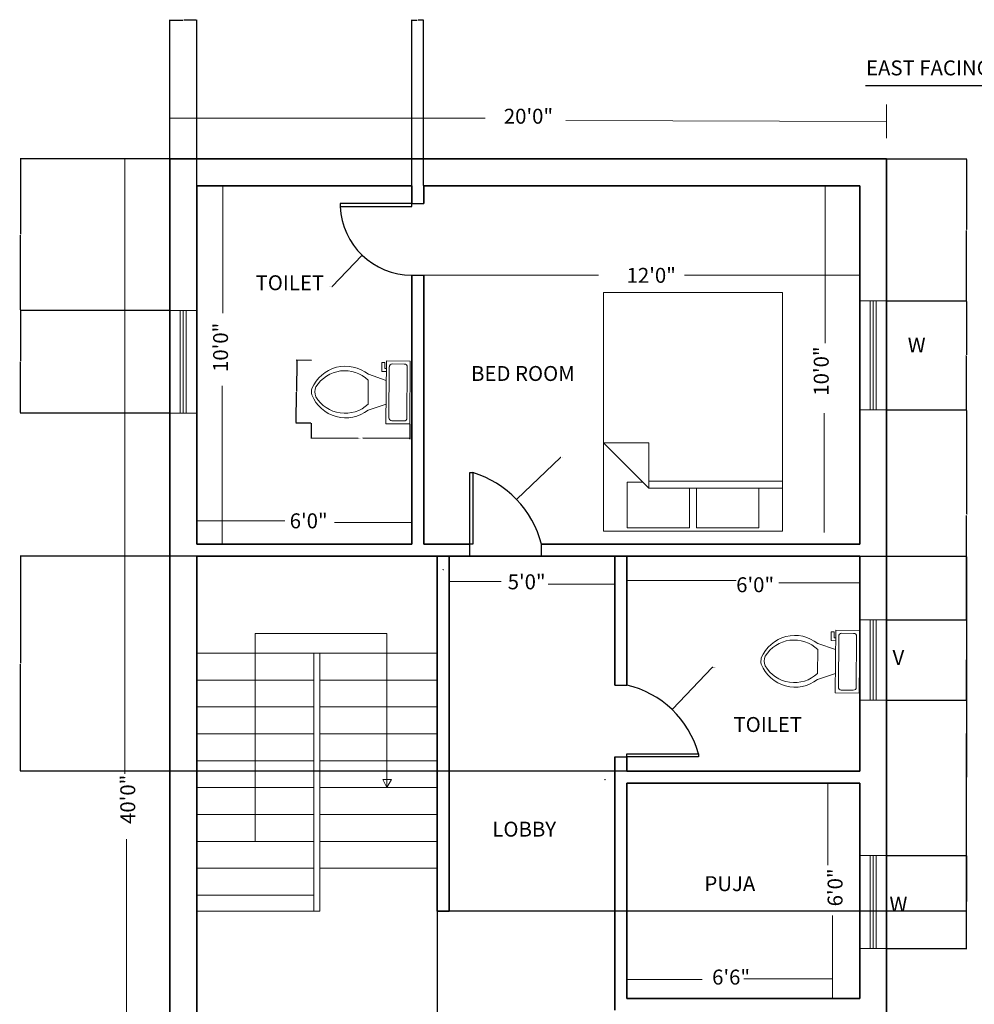
# Model space of a CAD drawing. Units: inches. Extents: x 37 to 686, y -425 to 128.
# Tile 2 of 3: x 37 to 357, y -201 to 128. Entities that reach past the tile are written whole.
import ezdxf

# ---------------------------------------------------------------- set-up
doc = ezdxf.new("R2010")
doc.units = ezdxf.units.IN
doc.header["$MEASUREMENT"] = 0
for name, color, linetype, lineweight in [('A-ANNO-DIMS', 2, 'Continuous', 13), ('A-ANNO-SYMB', 7, 'Continuous', 13), ('A-ANNO-TEXT', 7, 'Continuous', 18), ('A-ANNO-TITL', 7, 'Continuous', 25), ('A-AREA-IDEN', 7, 'Continuous', 18), ('A-DOOR', 3, 'Continuous', 25), ('A-FLOR-FIXT', 9, 'Continuous', 18), ('A-FLOR-STRS', 7, 'Continuous', 20), ('A-FURN', 8, 'Continuous', 18), ('A-GLAZ', 4, 'Continuous', 18), ('A-WALL', 7, 'Continuous', 35)]:
    doc.layers.add(name, color=color, linetype=linetype, lineweight=lineweight)
doc.styles.get("Standard").update_dxf_attribs({"font": 'arial.ttf'})
doc.dimstyles.get("Standard").update_dxf_attribs({"dimtxt": 0.18, "dimasz": 0.18, "dimexe": 0.18, "dimexo": 0.0625, "dimgap": 0.09, "dimtad": 0, "dimtih": 1, "dimtoh": 1, "dimdec": 4, "dimzin": 0, "dimdsep": 46, "dimtxsty": 'Standard', "dimcen": 0.09, "dimadec": 0, "dimazin": 0, "dimtfac": 1, "dimtdec": 4, "dimtofl": 0, "dimtmove": 0, "dimatfit": 3, "dimfxl": 1, "dimtolj": 1, "dimtzin": 0, "dimarcsym": 0})

# ---------------------------------------------------------------- blocks, each defined once
blk = doc.blocks.new('Toilet - top')
for p, q in [((9.5, -6), (9.5, -2)), ((-10, -8.5), (-8, -8.5)), ((-10, -9.5), (-10, -8.5)), ((-7, -9.5), (-10, -9.5)), ((-8, -8.5), (-8, -8)), ((-7, -8), (-7, -9.5)), ((-4, -8), (-6, -14)), ((4, -8), (6, -14)), ((4, -14), (-4, -14))]:
    blk.add_line(p, q)
blk.add_lwpolyline([(10.5, -8), (10.5, 0), (-10.5, 0), (-10.5, -8)], close=True)
for points in [[(-9.5, -2), (-9.5, -6)], [(8.5, -1), (-8.5, -1)], [(-8.5, -7), (8.5, -7)]]:
    blk.add_lwpolyline(points)
for centre, radius, start, end in [((-8.62, -1.88), 0.884, 81.8699, 188.1301), ((8.62, -1.88), 0.884, 351.8699, 98.1301), ((-8.62, -6.12), 0.884, 171.8699, 278.1301), ((8.62, -6.12), 0.884, 261.8699, 8.1301), ((3.52, -21.58), 12.17, 141.4691, 247.9714), ((4.2, -21.82), 11.33, 136.3677, 238.9468), ((-3.52, -21.58), 12.17, 292.0284, 38.5307), ((-4.2, -21.82), 11.33, 301.053, 43.6321), ((0, -27.88), 4, 245.7318, 294.2682), ((0, -29), 4, 254.8605, 285.1395)]:
    blk.add_arc(centre, radius, start, end)
blk = doc.blocks.new('Bed - Queen')
for p, q in [((0, -80.00003), (0, 0)), ((0, 0), (59.99999, 0)), ((59.99999, 0), (59.99999, -80.00003)), ((7.99999, -1.2), (28.79998, -1.2)), ((7.99999, -14.4), (7.99999, -1.2)), ((28.79998, -1.2), (28.79998, -14.4)), ((31.19999, -1.2), (51.99999, -1.2)), ((31.19999, -14.4), (31.19999, -1.2)), ((51.99999, -1.2), (51.99999, -16.4)), ((0, -14.4), (44.8, -14.4)), ((59.99999, -29.6), (44.8, -14.4)), ((44.8, -14.4), (44.8, -29.6)), ((51.99999, -16.4), (46.79936, -16.4)), ((44.8, -16.8), (0, -16.8)), ((44.8, -29.6), (59.99999, -29.6)), ((59.99999, -80.00003), (0, -80.00003))]:
    blk.add_line(p, q)
blk = doc.blocks.new('DOOR-LEAF-24IN')
for p, q in [((0, 0), (0, 24)), ((0, 24), (1, 24)), ((1, 24), (1, 0)), ((1, 0), (0, 0))]:
    blk.add_line(p, q)
blk = doc.blocks.new('*D10')
at = {"layer": 'A-ANNO-DIMS', "color": 0, "lineweight": -2, "transparency": 16777216}
for p, q in [((134.95, -6.72), (134.91, -11.8)), ((167.99, -6.97), (167.95, -12.04)), ((135.09, -11.62), (150.66, -11.73)), ((167.77, -11.86), (152.21, -11.75))]:
    blk.add_line(p, q, dxfattribs=at)
at = {"layer": 'A-ANNO-DIMS', "color": 0, "transparency": 16777216}
for points in [[(135.09, -11.59), (135.09, -11.65), (134.91, -11.62)], [(167.77, -11.83), (167.77, -11.89), (167.95, -11.86)]]:
    blk.add_solid(points, dxfattribs=at)
at = {"layer": 'Defpoints', "color": 0, "transparency": 16777216}
for p in [(134.95, -6.66), (167.99, -6.91), (167.95, -11.86)]:
    blk.add_point(p, dxfattribs=at)
at = {"layer": 'A-ANNO-DIMS', "color": 0, "transparency": 16777216, "insert": (151.43, -11.74), "char_height": 0.18, "attachment_point": 5}
blk.add_mtext('\\A1;WC 33 TYP.', dxfattribs=at)
blk = doc.blocks.new('*D11')
at = {"layer": 'A-ANNO-DIMS', "color": 0, "lineweight": -2, "transparency": 16777216}
for p, q in [((135.04, 14.34), (129.97, 14.38)), ((130.14, 14.2), (130.07, 4.06)), ((129.99, -6.44), (130.07, 3.7)), ((134.88, -6.66), (129.81, -6.62))]:
    blk.add_line(p, q, dxfattribs=at)
at = {"layer": 'A-ANNO-DIMS', "color": 0, "transparency": 16777216}
for points in [[(130.11, 14.2), (130.17, 14.2), (130.15, 14.38)], [(129.96, -6.44), (130.02, -6.44), (129.99, -6.62)]]:
    blk.add_solid(points, dxfattribs=at)
at = {"layer": 'Defpoints', "color": 0, "transparency": 16777216}
for p in [(135.1, 14.34), (129.99, -6.62), (134.95, -6.66)]:
    blk.add_point(p, dxfattribs=at)
at = {"layer": 'A-ANNO-DIMS', "color": 0, "transparency": 16777216, "insert": (130.07, 3.88), "char_height": 0.18, "attachment_point": 5}
blk.add_mtext('\\A1;21 TYP.', dxfattribs=at)
blk = doc.blocks.new('*D22')
at = {"layer": 'A-ANNO-DIMS', "color": 0, "lineweight": -2, "transparency": 16777216}
for p, q in [((240.57, -51.23), (37.48, -51.23)), ((37.66, -51.41), (37.66, -87.05)), ((37.66, -123.05), (37.66, -87.41)), ((240.57, -123.23), (37.48, -123.23))]:
    blk.add_line(p, q, dxfattribs=at)
at = {"layer": 'A-ANNO-DIMS', "color": 0, "transparency": 16777216}
for points in [[(37.63, -51.41), (37.69, -51.41), (37.66, -51.23)], [(37.63, -123.05), (37.69, -123.05), (37.66, -123.23)]]:
    blk.add_solid(points, dxfattribs=at)
at = {"layer": 'Defpoints', "color": 0, "transparency": 16777216}
for p in [(240.63, -51.23), (37.66, -123.23), (240.63, -123.23)]:
    blk.add_point(p, dxfattribs=at)
at = {"layer": 'A-ANNO-DIMS', "color": 0, "transparency": 16777216, "insert": (37.66, -87.23), "char_height": 0.18, "attachment_point": 5}
blk.add_mtext('\\A1;72', dxfattribs=at)
blk = doc.blocks.new('*D23')
at = {"layer": 'A-ANNO-DIMS', "color": 0, "lineweight": -2, "transparency": 16777216}
for p, q in [((96.63, -51.29), (96.63, -425.16)), ((177.14, -51.29), (177.14, -425.16)), ((96.81, -424.98), (136.56, -424.98)), ((176.96, -424.98), (137.21, -424.98))]:
    blk.add_line(p, q, dxfattribs=at)
at = {"layer": 'A-ANNO-DIMS', "color": 0, "transparency": 16777216}
for points in [[(96.81, -424.95), (96.81, -425.01), (96.63, -424.98)], [(176.96, -424.95), (176.96, -425.01), (177.14, -424.98)]]:
    blk.add_solid(points, dxfattribs=at)
at = {"layer": 'Defpoints', "color": 0, "transparency": 16777216}
for p in [(96.63, -51.23), (177.14, -51.23), (177.14, -424.98)]:
    blk.add_point(p, dxfattribs=at)
at = {"layer": 'A-ANNO-DIMS', "color": 0, "transparency": 16777216, "insert": (136.88, -424.98), "char_height": 0.18, "attachment_point": 5}
blk.add_mtext('\\A1;80.5', dxfattribs=at)
blk = doc.blocks.new('*D29')
at = {"layer": 'A-ANNO-DIMS', "color": 0, "lineweight": -2, "transparency": 16777216}
for p, q in [((87.57, 31.06), (37.48, 31.06)), ((37.66, 30.88), (37.66, 14.07)), ((37.66, -3.11), (37.66, 13.71)), ((87.57, -3.29), (37.48, -3.29))]:
    blk.add_line(p, q, dxfattribs=at)
at = {"layer": 'A-ANNO-DIMS', "color": 0, "transparency": 16777216}
for points in [[(37.63, 30.88), (37.69, 30.88), (37.66, 31.06)], [(37.63, -3.11), (37.69, -3.11), (37.66, -3.29)]]:
    blk.add_solid(points, dxfattribs=at)
at = {"layer": 'Defpoints', "color": 0, "transparency": 16777216}
for p in [(37.66, 31.06), (87.63, 31.06), (87.63, -3.29)]:
    blk.add_point(p, dxfattribs=at)
at = {"layer": 'A-ANNO-DIMS', "color": 0, "transparency": 16777216, "insert": (37.66, 13.89), "char_height": 0.18, "attachment_point": 5}
blk.add_mtext('\\A1;34.35', dxfattribs=at)
blk = doc.blocks.new('*D30')
at = {"layer": 'A-ANNO-DIMS', "color": 0, "lineweight": -2, "transparency": 16777216}
for p, q in [((327.69, 34.28), (354.56, 34.28)), ((354.38, 34.1), (354.38, 16.22)), ((354.38, -2.03), (354.38, 15.85)), ((327.69, -2.21), (354.56, -2.21))]:
    blk.add_line(p, q, dxfattribs=at)
at = {"layer": 'A-ANNO-DIMS', "color": 0, "transparency": 16777216}
for points in [[(354.35, 34.1), (354.41, 34.1), (354.38, 34.28)], [(354.35, -2.03), (354.41, -2.03), (354.38, -2.21)]]:
    blk.add_solid(points, dxfattribs=at)
at = {"layer": 'Defpoints', "color": 0, "transparency": 16777216}
for p in [(327.63, 34.28), (354.38, 34.28), (327.63, -2.21)]:
    blk.add_point(p, dxfattribs=at)
at = {"layer": 'A-ANNO-DIMS', "color": 0, "transparency": 16777216, "insert": (354.38, 16.03), "char_height": 0.18, "attachment_point": 5}
blk.add_mtext('\\A1;36.496', dxfattribs=at)
blk = doc.blocks.new('*D33')
at = {"layer": 'A-ANNO-DIMS', "color": 0, "lineweight": -2, "transparency": 16777216}
for p, q in [((327.69, -151.36), (354.56, -151.36)), ((354.38, -151.54), (354.38, -166.74)), ((354.38, -182.31), (354.38, -167.11)), ((327.69, -182.49), (354.56, -182.49))]:
    blk.add_line(p, q, dxfattribs=at)
at = {"layer": 'A-ANNO-DIMS', "color": 0, "transparency": 16777216}
for points in [[(354.35, -151.54), (354.41, -151.54), (354.38, -151.36)], [(354.35, -182.31), (354.41, -182.31), (354.38, -182.49)]]:
    blk.add_solid(points, dxfattribs=at)
at = {"layer": 'Defpoints', "color": 0, "transparency": 16777216}
for p in [(327.63, -151.36), (354.38, -151.36), (327.63, -182.49)]:
    blk.add_point(p, dxfattribs=at)
at = {"layer": 'A-ANNO-DIMS', "color": 0, "transparency": 16777216, "insert": (354.38, -166.92), "char_height": 0.18, "attachment_point": 5}
blk.add_mtext('\\A1;31.13', dxfattribs=at)
blk = doc.blocks.new('*D34')
at = {"layer": 'A-ANNO-DIMS', "color": 0, "lineweight": -2, "transparency": 16777216}
for p, q in [((327.69, -72.53), (354.56, -72.53)), ((354.38, -72.71), (354.38, -85.76)), ((354.38, -99.18), (354.38, -86.13)), ((327.69, -99.36), (354.56, -99.36))]:
    blk.add_line(p, q, dxfattribs=at)
at = {"layer": 'A-ANNO-DIMS', "color": 0, "transparency": 16777216}
for points in [[(354.35, -72.71), (354.41, -72.71), (354.38, -72.53)], [(354.35, -99.18), (354.41, -99.18), (354.38, -99.36)]]:
    blk.add_solid(points, dxfattribs=at)
at = {"layer": 'Defpoints', "color": 0, "transparency": 16777216}
for p in [(327.63, -72.53), (354.38, -72.53), (327.63, -99.36)]:
    blk.add_point(p, dxfattribs=at)
at = {"layer": 'A-ANNO-DIMS', "color": 0, "transparency": 16777216, "insert": (354.38, -85.94), "char_height": 0.18, "attachment_point": 5}
blk.add_mtext('\\A1;26.835', dxfattribs=at)
blk = doc.blocks.new('*D41')
at = {"layer": 'A-ANNO-DIMS', "color": 0, "lineweight": -2, "transparency": 16777216}
for p, q in [((87.57, 81.77), (37.48, 81.77)), ((37.66, 81.59), (37.66, 56.6)), ((37.66, 31.24), (37.66, 56.24)), ((87.57, 31.06), (37.48, 31.06))]:
    blk.add_line(p, q, dxfattribs=at)
at = {"layer": 'A-ANNO-DIMS', "color": 0, "transparency": 16777216}
for points in [[(37.63, 81.59), (37.69, 81.59), (37.66, 81.77)], [(37.63, 31.24), (37.69, 31.24), (37.66, 31.06)]]:
    blk.add_solid(points, dxfattribs=at)
at = {"layer": 'Defpoints', "color": 0, "transparency": 16777216}
for p in [(87.63, 81.77), (37.66, 31.06), (87.63, 31.06)]:
    blk.add_point(p, dxfattribs=at)
at = {"layer": 'A-ANNO-DIMS', "color": 0, "transparency": 16777216, "insert": (37.66, 56.42), "char_height": 0.18, "attachment_point": 5}
blk.add_mtext('\\A1;50.71', dxfattribs=at)
blk = doc.blocks.new('*D42')
at = {"layer": 'A-ANNO-DIMS', "color": 0, "lineweight": -2, "transparency": 16777216}
for p, q in [((327.69, 81.77), (354.56, 81.77)), ((354.38, 81.59), (354.38, 58.21)), ((354.38, 34.46), (354.38, 57.85)), ((327.69, 34.28), (354.56, 34.28))]:
    blk.add_line(p, q, dxfattribs=at)
at = {"layer": 'A-ANNO-DIMS', "color": 0, "transparency": 16777216}
for points in [[(354.35, 81.59), (354.41, 81.59), (354.38, 81.77)], [(354.35, 34.46), (354.41, 34.46), (354.38, 34.28)]]:
    blk.add_solid(points, dxfattribs=at)
at = {"layer": 'Defpoints', "color": 0, "transparency": 16777216}
for p in [(327.63, 81.77), (327.63, 34.28), (354.38, 34.28)]:
    blk.add_point(p, dxfattribs=at)
at = {"layer": 'A-ANNO-DIMS', "color": 0, "transparency": 16777216, "insert": (354.38, 58.03), "char_height": 0.18, "attachment_point": 5}
blk.add_mtext('\\A1;47.49', dxfattribs=at)
blk = doc.blocks.new('*D45')
at = {"layer": 'A-ANNO-DIMS', "color": 0, "lineweight": -2, "transparency": 16777216}
for p, q in [((327.69, -99.36), (354.56, -99.36)), ((354.38, -99.54), (354.38, -125.18)), ((354.38, -151.18), (354.38, -125.54)), ((327.69, -151.36), (354.56, -151.36))]:
    blk.add_line(p, q, dxfattribs=at)
at = {"layer": 'A-ANNO-DIMS', "color": 0, "transparency": 16777216}
for points in [[(354.35, -99.54), (354.41, -99.54), (354.38, -99.36)], [(354.35, -151.18), (354.41, -151.18), (354.38, -151.36)]]:
    blk.add_solid(points, dxfattribs=at)
at = {"layer": 'Defpoints', "color": 0, "transparency": 16777216}
for p in [(327.63, -99.36), (354.38, -99.36), (327.63, -151.36)]:
    blk.add_point(p, dxfattribs=at)
at = {"layer": 'A-ANNO-DIMS', "color": 0, "transparency": 16777216, "insert": (354.38, -125.36), "char_height": 0.18, "attachment_point": 5}
blk.add_mtext('\\A1;52', dxfattribs=at)
blk = doc.blocks.new('*D46')
at = {"layer": 'A-ANNO-DIMS', "color": 0, "lineweight": -2, "transparency": 16777216}
for p, q in [((327.69, -2.21), (354.56, -2.21)), ((354.38, -2.39), (354.38, -37.19)), ((354.38, -72.35), (354.38, -37.55)), ((327.69, -72.53), (354.56, -72.53))]:
    blk.add_line(p, q, dxfattribs=at)
at = {"layer": 'A-ANNO-DIMS', "color": 0, "transparency": 16777216}
for points in [[(354.35, -2.39), (354.41, -2.39), (354.38, -2.21)], [(354.35, -72.35), (354.41, -72.35), (354.38, -72.53)]]:
    blk.add_solid(points, dxfattribs=at)
at = {"layer": 'Defpoints', "color": 0, "transparency": 16777216}
for p in [(327.63, -2.21), (354.38, -2.21), (327.63, -72.53)]:
    blk.add_point(p, dxfattribs=at)
at = {"layer": 'A-ANNO-DIMS', "color": 0, "transparency": 16777216, "insert": (354.38, -37.37), "char_height": 0.18, "attachment_point": 5}
blk.add_mtext('\\A1;70.31', dxfattribs=at)
blk = doc.blocks.new('*D57')
at = {"layer": 'A-ANNO-DIMS', "color": 0, "lineweight": -2, "transparency": 16777216}
for p, q in [((177.2, -51.23), (354.56, -51.23)), ((354.38, -51.41), (354.38, -110.43)), ((354.38, -169.81), (354.38, -110.79)), ((177.2, -169.99), (354.56, -169.99))]:
    blk.add_line(p, q, dxfattribs=at)
at = {"layer": 'A-ANNO-DIMS', "color": 0, "transparency": 16777216}
for points in [[(354.35, -51.41), (354.41, -51.41), (354.38, -51.23)], [(354.35, -169.81), (354.41, -169.81), (354.38, -169.99)]]:
    blk.add_solid(points, dxfattribs=at)
at = {"layer": 'Defpoints', "color": 0, "transparency": 16777216}
for p in [(177.14, -51.23), (354.38, -51.23), (177.14, -169.99)]:
    blk.add_point(p, dxfattribs=at)
at = {"layer": 'A-ANNO-DIMS', "color": 0, "transparency": 16777216, "insert": (354.38, -110.61), "char_height": 0.18, "attachment_point": 5}
blk.add_mtext('\\A1;118.76', dxfattribs=at)
blk = doc.blocks.new('*D58')
at = {"layer": 'A-ANNO-DIMS', "color": 0, "lineweight": -2, "transparency": 16777216}
for p, q in [((87.63, 81.84), (87.63, 128.4)), ((87.81, 128.22), (91.98, 128.22)), ((96.45, 128.22), (92.28, 128.22)), ((96.63, 72.84), (96.63, 128.4))]:
    blk.add_line(p, q, dxfattribs=at)
at = {"layer": 'A-ANNO-DIMS', "color": 0, "transparency": 16777216}
for points in [[(87.81, 128.25), (87.81, 128.19), (87.63, 128.22)], [(96.45, 128.25), (96.45, 128.19), (96.63, 128.22)]]:
    blk.add_solid(points, dxfattribs=at)
at = {"layer": 'Defpoints', "color": 0, "transparency": 16777216}
for p in [(96.63, 128.22), (87.63, 81.77), (96.63, 72.77)]:
    blk.add_point(p, dxfattribs=at)
at = {"layer": 'A-ANNO-DIMS', "color": 0, "transparency": 16777216, "insert": (92.13, 128.22), "char_height": 0.18, "attachment_point": 5}
blk.add_mtext('\\A1;9', dxfattribs=at)
blk = doc.blocks.new('*D59')
at = {"layer": 'A-ANNO-DIMS', "color": 0, "lineweight": -2, "transparency": 16777216}
for p, q in [((168.63, 72.84), (168.63, 128.4)), ((168.81, 128.22), (170.48, 128.22)), ((172.45, 128.22), (170.78, 128.22)), ((172.63, 72.84), (172.63, 128.4))]:
    blk.add_line(p, q, dxfattribs=at)
at = {"layer": 'A-ANNO-DIMS', "color": 0, "transparency": 16777216}
for points in [[(168.81, 128.25), (168.81, 128.19), (168.63, 128.22)], [(172.45, 128.25), (172.45, 128.19), (172.63, 128.22)]]:
    blk.add_solid(points, dxfattribs=at)
at = {"layer": 'Defpoints', "color": 0, "transparency": 16777216}
for p in [(172.63, 128.22), (168.63, 72.77), (172.63, 72.77)]:
    blk.add_point(p, dxfattribs=at)
at = {"layer": 'A-ANNO-DIMS', "color": 0, "transparency": 16777216, "insert": (170.63, 128.22), "char_height": 0.18, "attachment_point": 5}
blk.add_mtext('\\A1;4', dxfattribs=at)
blk = doc.blocks.new('*D62')
at = {"layer": 'A-ANNO-DIMS', "color": 0, "lineweight": -2, "transparency": 16777216}
for p, q in [((218.42, -18.12), (203.84, -32.1)), ((218.6, -18.12), (218.42, -18.12)), ((179.11, -55.71), (179.29, -55.71)), ((179.2, -55.8), (179.2, -55.62))]:
    blk.add_line(p, q, dxfattribs=at)
at = {"layer": 'A-ANNO-DIMS', "color": 0, "transparency": 16777216}
blk.add_solid([(203.82, -32.07), (203.87, -32.12), (203.72, -32.22)], dxfattribs=at)
at = {"layer": 'Defpoints', "color": 0, "transparency": 16777216}
for p in [(203.72, -32.22), (179.2, -55.71)]:
    blk.add_point(p, dxfattribs=at)
at = {"layer": 'A-ANNO-DIMS', "color": 0, "transparency": 16777216, "insert": (219.08, -18.12), "char_height": 0.18, "attachment_point": 5}
blk.add_mtext('\\A1;R33.95', dxfattribs=at)
blk = doc.blocks.new('*D64')
at = {"layer": 'A-ANNO-DIMS', "color": 0, "lineweight": -2, "transparency": 16777216}
for p, q in [((269.26, -88.51), (255.93, -102.42)), ((269.44, -88.51), (269.26, -88.51)), ((233.28, -125.96), (233.46, -125.96)), ((233.37, -126.05), (233.37, -125.87))]:
    blk.add_line(p, q, dxfattribs=at)
at = {"layer": 'A-ANNO-DIMS', "color": 0, "transparency": 16777216}
blk.add_solid([(255.91, -102.4), (255.95, -102.44), (255.8, -102.55)], dxfattribs=at)
at = {"layer": 'Defpoints', "color": 0, "transparency": 16777216}
for p in [(255.8, -102.55), (233.37, -125.96)]:
    blk.add_point(p, dxfattribs=at)
at = {"layer": 'A-ANNO-DIMS', "color": 0, "transparency": 16777216, "insert": (269.92, -88.51), "char_height": 0.18, "attachment_point": 5}
blk.add_mtext('\\A1;R32.42', dxfattribs=at)
blk = doc.blocks.new('*D68')
at = {"layer": 'A-ANNO-DIMS', "color": 0, "lineweight": -2, "transparency": 16777216}
for p, q in [((168.74, 67.06), (168.92, 67.06)), ((168.83, 66.97), (168.83, 67.15)), ((142.01, 39.06), (151.94, 49.43)), ((141.83, 39.06), (142.01, 39.06))]:
    blk.add_line(p, q, dxfattribs=at)
at = {"layer": 'A-ANNO-DIMS', "color": 0, "transparency": 16777216}
blk.add_solid([(151.92, 49.45), (151.96, 49.41), (152.07, 49.56)], dxfattribs=at)
at = {"layer": 'Defpoints', "color": 0, "transparency": 16777216}
for p in [(168.83, 67.06), (152.07, 49.56)]:
    blk.add_point(p, dxfattribs=at)
at = {"layer": 'A-ANNO-DIMS', "color": 0, "transparency": 16777216, "insert": (141.28, 39.06), "char_height": 0.18, "attachment_point": 5}
blk.add_mtext('\\A1;R24.234', dxfattribs=at)

msp = doc.modelspace()

# ---------------------------------------------------------------- linework, layer by layer
at = {"layer": 'A-ANNO-DIMS'}
for p, q in [((87.6318, 89.3296), (87.6318, 101.4672)), ((327.6318, 88.7375), (327.6318, 99.987)), ((87.6318, 95.3984), (193.251, 95.3984)), ((220.2222, 94.6583), (327.6318, 94.3623)), ((80.7552, 81.7729), (64.4114, 81.7729)), ((72.5833, 81.7729), (72.5833, -124.1157)), ((105.4086, 30.1915), (105.4086, 72.7729)), ((307.0425, 72.7729), (307.0425, 30.3669)), ((172.6318, 42.8225), (231.1891, 42.8225)), ((259.9386, 42.8225), (318.6318, 42.8225)), ((307.0425, 30.3669), (307.0425, 20.1003)), ((105.1115, 5.8627), (105.1115, -47.2271)), ((306.7951, -3.3013), (306.7951, -43.2278)), ((96.6318, -39.3418), (126.118, -39.3418)), ((142.7992, -39.9243), (168.6318, -39.9243)), ((181.1379, -59.6558), (198.6356, -59.6558)), ((214.275, -60.6092), (236.6318, -60.6092)), ((240.6318, -59.3672), (277.2772, -59.3672)), ((291.6142, -60.0741), (318.6318, -60.0741)), ((307.994, -127.2271), (307.994, -154.6672)), ((73.1317, -145.9359), (73.1317, -398.2271)), ((309.5265, -171.5046), (309.5265, -199.2271)), ((240.6318, -192.9341), (265.8511, -192.9341)), ((279.8349, -192.7428), (309.5265, -192.7428))]:
    msp.add_line(p, q, dxfattribs=at)
at = {"layer": 'A-ANNO-SYMB'}
for p, q in [((116.2583, -146.6754), (116.2583, -77.1163)), ((116.2583, -77.1163), (160.3362, -77.1163)), ((160.3362, -77.1163), (160.3362, -128.6754)), ((158.9278, -125.973), (161.814, -125.973)), ((160.2537, -128.6754), (158.9278, -125.973)), ((161.814, -125.973), (160.2537, -128.6754))]:
    msp.add_line(p, q, dxfattribs=at)
at = {"layer": 'A-ANNO-TITL'}
msp.add_line((320.568, 106.3633), (393.4497, 106.3633), dxfattribs=at)
at = {"layer": 'A-DOOR'}
for p, q in [((168.6318, 66.8225), (144.6318, 66.8225)), ((144.6318, 66.8225), (144.6318, 65.8225)), ((168.6318, 65.8225), (168.6318, 67.4973)), ((168.6318, 66.8225), (172.6318, 66.8225)), ((144.6318, 65.8225), (168.6318, 65.8225)), ((168.6318, 42.8225), (172.6318, 42.8225)), ((188.0768, -51.2271), (188.0768, -47.2271)), ((212.0768, -51.2271), (212.0768, -47.2271)), ((236.6318, -94.361), (240.6318, -94.361)), ((236.6318, -118.361), (240.6318, -118.361))]:
    msp.add_line(p, q, dxfattribs=at)
for centre, radius, start, end in [((168.8344, 67.0557), 24.234, 182.916723, 269.521028), ((179.2016, -55.7117), 33.9524, 14.471364, 73.090885), ((233.3707, -125.9595), 32.4221, 15.379189, 77.058561)]:
    msp.add_arc(centre, radius, start, end, dxfattribs=at)
at = {"layer": 'A-FLOR-STRS'}
for p, q in [((177.1379, -83.6754), (96.6318, -83.6754)), ((135.8849, -169.9919), (135.8849, -83.6754)), ((137.8849, -169.9919), (137.8849, -83.6754)), ((135.8849, -92.6754), (96.6318, -92.6754)), ((177.1379, -92.6754), (137.8849, -92.6754)), ((135.8849, -101.6754), (96.6318, -101.6754)), ((177.1379, -101.6754), (137.8849, -101.6754)), ((135.8849, -110.6754), (96.6318, -110.6754)), ((177.1379, -110.6754), (137.8849, -110.6754)), ((135.8849, -119.6754), (96.6318, -119.6754)), ((177.1379, -119.6754), (137.8849, -119.6754)), ((135.8849, -128.6754), (96.6318, -128.6754)), ((177.1379, -128.6754), (137.8849, -128.6754)), ((135.8849, -137.6754), (96.6318, -137.6754)), ((177.1379, -137.6754), (137.8849, -137.6754)), ((135.8849, -146.6754), (96.6318, -146.6754)), ((177.1379, -146.6754), (137.8849, -146.6754)), ((135.8849, -155.6754), (96.6318, -155.6754)), ((177.1379, -155.6754), (137.8849, -155.6754)), ((135.8849, -164.6754), (96.6318, -164.6754)), ((137.8849, -169.9919), (96.6318, -169.9919))]:
    msp.add_line(p, q, dxfattribs=at)
at = {"layer": 'A-GLAZ'}
for p, q in [((318.6318, 34.2824), (327.6318, 34.2824)), ((322.1318, 34.2824), (322.1318, -2.2137)), ((323.1318, 34.2824), (323.1318, -2.2137)), ((324.1318, 34.2824), (324.1318, -2.2137)), ((87.6318, 31.0642), (96.6318, 31.0642)), ((91.1318, 31.0642), (91.1318, -3.2851)), ((92.1318, 31.0642), (92.1318, -3.2851)), ((93.1318, 31.0642), (93.1318, -3.2851)), ((87.6318, -3.2851), (96.6318, -3.2851)), ((318.6318, -2.2137), (327.6318, -2.2137)), ((318.6318, -72.5261), (327.6318, -72.5261)), ((322.1318, -72.5261), (322.1318, -99.3614)), ((323.1318, -72.5261), (323.1318, -99.3614)), ((324.1318, -72.5261), (324.1318, -99.3614)), ((318.6318, -99.3614), (327.6318, -99.3614)), ((318.6318, -151.3603), (327.6318, -151.3603)), ((322.1318, -151.3603), (322.1318, -182.4893)), ((323.1318, -151.3603), (323.1318, -182.4893)), ((324.1318, -151.3603), (324.1318, -182.4893)), ((318.6318, -182.4893), (327.6318, -182.4893))]:
    msp.add_line(p, q, dxfattribs=at)
at = {"layer": 'A-WALL'}
for p, q in [((96.6318, 72.7729), (168.6318, 72.7729)), ((96.6318, -47.2271), (96.6318, 72.7729)), ((168.6318, 66.8225), (168.6318, 72.7729)), ((172.6318, 66.8225), (172.6318, 72.7729)), ((172.6318, 72.7729), (318.6318, 72.7729)), ((318.6318, 72.7729), (318.6318, -47.2271)), ((168.6318, -47.2271), (168.6318, 42.8225)), ((172.6318, -47.2271), (172.6318, 42.8225)), ((96.6318, -47.2271), (168.6318, -47.2271)), ((172.6318, -47.2271), (188.0768, -47.2271)), ((212.0768, -47.2271), (318.6318, -47.2271)), ((96.6318, -389.2271), (96.6318, -51.2271)), ((96.6318, -51.2271), (177.1379, -51.2271)), ((177.1379, -51.2271), (177.1379, -153.2802)), ((181.1379, -51.2271), (181.1379, -153.2802)), ((181.1379, -51.2271), (188.0768, -51.2271)), ((212.0768, -51.2271), (236.6318, -51.2271)), ((236.6318, -51.2271), (236.6318, -94.361)), ((240.6318, -51.2271), (240.6318, -94.361)), ((240.6318, -51.2271), (318.6318, -51.2271)), ((318.6318, -51.2271), (318.6318, -123.2271)), ((236.6318, -118.361), (236.6318, -203.2271)), ((240.6318, -118.361), (240.6318, -123.2271)), ((240.6318, -123.2271), (318.6318, -123.2271)), ((240.6318, -127.2271), (318.6318, -127.2271)), ((240.6318, -127.2271), (240.6318, -199.2271)), ((318.6318, -127.2271), (318.6318, -199.2271)), ((177.1379, -153.2802), (177.1379, -169.9919)), ((181.1379, -169.9919), (181.1379, -153.2802)), ((177.1379, -169.9919), (181.1379, -169.9919)), ((240.6318, -199.2271), (318.6318, -199.2271))]:
    msp.add_line(p, q, dxfattribs=at)
msp.add_lwpolyline([(87.6318, 81.7729), (327.6318, 81.7729), (327.6318, -398.2271), (87.6318, -398.2271)], close=True, dxfattribs=at)

# ---------------------------------------------------------------- block references
at = {"layer": 'A-DOOR'}
msp.add_blockref('DOOR-LEAF-24IN', (188.077, -47.227), dxfattribs=at)
at = {"layer": 'A-DOOR', "rotation": 89.99999999999991}
msp.add_blockref('DOOR-LEAF-24IN', (264.6317, -118.3608), dxfattribs=at)
at = {"layer": 'A-FLOR-FIXT', "rotation": 269.5733184257299}
for p in [(168.0698, 3.5942), (318.5536, -86.558)]:
    msp.add_blockref('Toilet - top', p, dxfattribs=at)
at = {"layer": 'A-FURN', "rotation": 180}
msp.add_blockref('Bed - Queen', (292.8168, -42.8782), dxfattribs=at)

# ---------------------------------------------------------------- texts
at = {"layer": 'A-ANNO-DIMS', "char_height": 5, "attachment_point": 1}
for s, width, insert in [('20\'0"', 66.49393, (199.4751, 98.5799)), ('12\'0"', 35.858568, (240.5954, 45.3112)), ('6\'0"', 27.670391, (127.7758, -36.8746)), ('5\'0"', 20.747672, (200.7652, -57.2907)), ('6\'0"', 27.670391, (277.2772, -58.2717)), ('6\'6"', 30.841433, (269.2204, -189.619))]:
    msp.add_mtext_dynamic_manual_height_columns(s, width=width, gutter_width=25, heights=[0], dxfattribs=dict(at, insert=insert))
at = {"layer": 'A-ANNO-DIMS', "char_height": 5, "attachment_point": 1, "rotation": 90}
for s, width, insert in [('10\'0"', 27.842625, (102.1156, 10.4667)), ('10\'0"', 27.842625, (303.2568, 2.5243)), ('40\'0"', 31.535776, (71.0496, -140.8477)), ('6\'0"', 27.670391, (307.9005, -168.4409))]:
    msp.add_mtext_dynamic_manual_height_columns(s, width=width, gutter_width=25, heights=[0], dxfattribs=dict(at, insert=insert))
at = {"layer": 'A-ANNO-TEXT', "char_height": 5, "attachment_point": 1}
for s, width, insert in [('W', 14.305566, (334.722, 22.0003)), ('V', 13.447234, (329.6363, -82.6031)), ('W', 8.568355, (328.6141, -165.2002))]:
    msp.add_mtext_dynamic_manual_height_columns(s, width=width, gutter_width=25, heights=[0], dxfattribs=dict(at, insert=insert))
at = {"layer": 'A-ANNO-TITL', "insert": (320.7609, 114.7635), "char_height": 5, "attachment_point": 1}
msp.add_mtext_dynamic_manual_height_columns('EAST FACING HOUSE', width=258.611498, gutter_width=25, heights=[0], dxfattribs=at)
at = {"layer": 'A-AREA-IDEN', "char_height": 5, "attachment_point": 1}
for s, width, insert in [('TOILET', 38.596876, (116.3431, 42.832)), ('BED ROOM', 83.955241, (188.5088, 12.4565)), ('TOILET', 38.596876, (276.3701, -105.0553)), ('LOBBY', 26.091096, (195.6274, -140.0935)), ('PUJA', 50.455237, (266.6459, -158.3351))]:
    msp.add_mtext_dynamic_manual_height_columns(s, width=width, gutter_width=25, heights=[0], dxfattribs=dict(at, insert=insert))

# ---------------------------------------------------------------- dimensions: what is measured, and where the dimension line sits
at = {"layer": 'A-ANNO-DIMS'}
for base, p1, p2, override, picture, middle in [((96.6318, 128.2172), (87.6318, 81.7729), (96.6318, 72.7729), {"dimdec": 0, "dimlfac": 1, "dimrnd": 0, "dimzin": 0, "dimdsep": 46, "dimlunit": 2}, '*D58', (92.1318, 128.2172)), ((172.6318, 128.2172), (168.6318, 72.7729), (172.6318, 72.7729), {"dimdec": 0, "dimlfac": 1, "dimrnd": 0, "dimzin": 0, "dimdsep": 46, "dimlunit": 2}, '*D59', (170.6318, 128.2172)), ((177.1379, -424.9771), (96.6318, -51.2271), (177.1379, -51.2271), {"dimdec": 1, "dimlfac": 1, "dimrnd": 0, "dimzin": 0, "dimdsep": 46, "dimlunit": 2}, '*D23', (136.8849, -424.9771))]:
    dim = msp.add_linear_dim(base=base, p1=p1, p2=p2, dimstyle='Standard', override=override, dxfattribs=at)
    dim.commit()
    dim.dimension.update_dxf_attribs({"geometry": picture, "text_midpoint": middle})
for base, p1, p2, override, picture, middle in [((37.6614, 31.0642), (87.6318, 81.7729), (87.6318, 31.0642), {"dimdec": 2, "dimlfac": 1, "dimrnd": 0, "dimzin": 0, "dimdsep": 46, "dimlunit": 2}, '*D41', (37.6614, 56.4185)), ((354.3818, 34.2824), (327.6318, 81.7729), (327.6318, 34.2824), {"dimdec": 2, "dimlfac": 1, "dimrnd": 0, "dimzin": 0, "dimdsep": 46, "dimlunit": 2}, '*D42', (354.3818, 58.0276)), ((354.3818, 34.2824), (327.6318, -2.2137), (327.6318, 34.2824), {"dimdec": 3, "dimlfac": 1, "dimrnd": 0, "dimzin": 0, "dimdsep": 46, "dimlunit": 2}, '*D30', (354.3818, 16.0343)), ((37.6614, 31.0642), (87.6318, -3.2851), (87.6318, 31.0642), {"dimdec": 2, "dimlfac": 1, "dimrnd": 0, "dimzin": 0, "dimdsep": 46, "dimlunit": 2}, '*D29', (37.6614, 13.8895)), ((354.3818, -2.2137), (327.6318, -72.5261), (327.6318, -2.2137), {"dimdec": 2, "dimlfac": 1, "dimrnd": 0, "dimzin": 0, "dimdsep": 46, "dimlunit": 2}, '*D46', (354.3818, -37.3699)), ((37.6614, -123.2271), (240.6318, -51.2271), (240.6318, -123.2271), {"dimdec": 0, "dimlfac": 1, "dimrnd": 0, "dimzin": 0, "dimdsep": 46, "dimlunit": 2}, '*D22', (37.6614, -87.2271)), ((354.3818, -51.2271), (177.1379, -169.9919), (177.1379, -51.2271), {"dimdec": 2, "dimlfac": 1, "dimrnd": 0, "dimzin": 0, "dimdsep": 46, "dimlunit": 2}, '*D57', (354.3818, -110.6095)), ((354.3818, -72.5261), (327.6318, -99.3614), (327.6318, -72.5261), {"dimdec": 3, "dimlfac": 1, "dimrnd": 0, "dimzin": 0, "dimdsep": 46, "dimlunit": 2}, '*D34', (354.3818, -85.9438)), ((354.3818, -99.3614), (327.6318, -151.3603), (327.6318, -99.3614), {"dimdec": 0, "dimlfac": 1, "dimrnd": 0, "dimzin": 0, "dimdsep": 46, "dimlunit": 2}, '*D45', (354.3818, -125.3609)), ((354.3818, -151.3603), (327.6318, -182.4893), (327.6318, -151.3603), {"dimdec": 2, "dimlfac": 1, "dimrnd": 0, "dimzin": 0, "dimdsep": 46, "dimlunit": 2}, '*D33', (354.3818, -166.9248))]:
    dim = msp.add_linear_dim(base=base, p1=p1, p2=p2, angle=90, dimstyle='Standard', override=override, dxfattribs=at)
    dim.commit()
    dim.dimension.update_dxf_attribs({"geometry": picture, "text_midpoint": middle})
for center, mpoint, override, picture, middle in [((168.8344, 67.0557), (152.0669, 49.5589), {"dimdec": 3, "dimlfac": 1, "dimrnd": 0, "dimzin": 0, "dimdsep": 46, "dimlunit": 2}, '*D68', (141.277, 39.0608)), ((179.2016, -55.7117), (203.715, -32.22), {"dimdec": 2, "dimlfac": 1, "dimrnd": 0, "dimzin": 0, "dimdsep": 46, "dimlunit": 2}, '*D62', (219.0836, -18.125)), ((233.3707, -125.9595), (255.8038, -102.5512), {"dimdec": 2, "dimlfac": 1, "dimrnd": 0, "dimzin": 0, "dimdsep": 46, "dimlunit": 2}, '*D64', (269.9225, -88.5063))]:
    dim = msp.add_radius_dim(center=center, mpoint=mpoint, dimstyle='Standard', override=override, dxfattribs=at)
    dim.commit()
    dim.dimension.update_dxf_attribs({"geometry": picture, "text_midpoint": middle, "dimtype": 164})
for base, p1, p2, angle, text, picture, middle in [((129.9895, -6.6225), (135.1026, 14.34), (134.9462, -6.6594), 269.573318, '<> TYP.', '*D11', (130.0676, 3.8772)), ((167.9547, -11.8623), (134.9462, -6.6594), (167.9916, -6.9055), 359.573318, 'WC <> TYP.', '*D10', (151.432, -11.7393))]:
    dim = msp.add_linear_dim(base=base, p1=p1, p2=p2, angle=angle, text=text, dimstyle='Standard', override={"dimdec": 0, "dimlfac": 1, "dimrnd": 0, "dimzin": 0, "dimdsep": 46, "dimlunit": 2}, dxfattribs=at)
    dim.commit()
    dim.dimension.update_dxf_attribs({"geometry": picture, "text_midpoint": middle})

doc.saveas('drawing.dxf')
